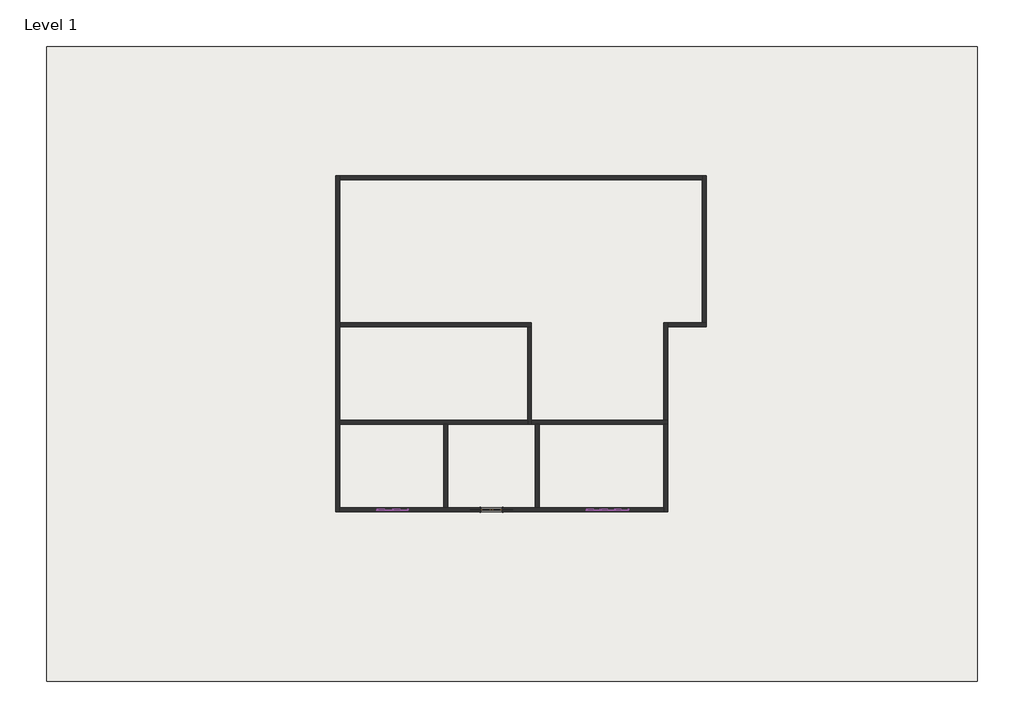
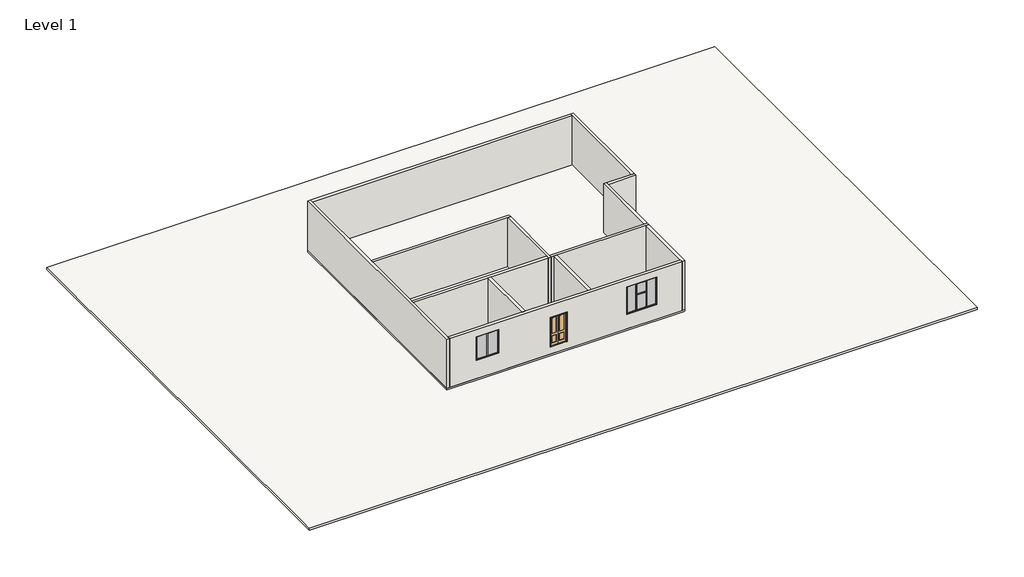
# One storey, incomplete: 22 members, 13 walls, 6 plates, 2 slabs, 1 door.
"""IFC4 building model written with IfcOpenShell, lengths in millimetres."""

from ifc_helpers import new_model, si_unit, frame, origin, origin_with_axes, place, context, project, spatial, polyline, outline, extrude, faceted_brep, transform, mapped, element, save
from components import door_interior_double_pocket_2_panel_wood_4_x_8_12c354ae, member_7007ad49, member_824a4a8d, member_798d6cad, member_9d02be77, member_c6627131, member_c17f1be2, member_f95d5bf5, member_18e22e2d, member_9193c932, member_0a82c195, system_panel_glazed_0771ef41, system_panel_glazed_b8cd24f7, system_panel_glazed_9a0fbd8e, system_panel_glazed_a3e6f34c

model = new_model("IFC4")

# Units and contexts
model_context = context("Model", 3, world=origin())
ifc_project = project(units=[si_unit("LENGTHUNIT", "METRE", prefix="MILLI")], contexts=[model_context])

# Site, building, storey
site = spatial("IfcSite", under=ifc_project)
building = spatial("IfcBuilding", under=site)
storey = spatial("IfcBuildingStorey", under=building, Name="Level 1", Elevation=0.0)

# Door
placement = place(None, origin())
door_interior_double_pocket_2_panel_wood_4_x_8_shape = door_interior_double_pocket_2_panel_wood_4_x_8_12c354ae(model_context)
element("IfcDoor", 1, ObjectType="Door-Interior-Double-Pocket-2_Panel-Wood : 4'x 8'", at=placement, inside=storey, context=model_context, shape_type="MappedRepresentation", body=[
    mapped(door_interior_double_pocket_2_panel_wood_4_x_8_shape, transform((-4678.5559085, -2978.2585517, 609.6), x_axis=(-1.0, 0.0, 0.0), y_axis=(0.0, -1.0, 0.0), z_axis=(0.0, 0.0, 1.0))),
])

# Members
member_shape = member_7007ad49(model_context)
element("IfcMember", 2, ObjectType="Rectangular Mullion : 2.5\" x 5\" rectangular", at=placement, inside=storey, context=model_context, shape_type="MappedRepresentation", body=[
    mapped(member_shape, transform((852.2940915, -2978.2585517, 3556.0), x_axis=(0.0, 0.0, 1.0), y_axis=(0.0, 1.0, 0.0), z_axis=(-1.0, 0.0, 0.0))),
])
element("IfcMember", 3, ObjectType="Rectangular Mullion : 2.5\" x 5\" rectangular", at=placement, inside=storey, context=model_context, shape_type="MappedRepresentation", body=[
    mapped(member_shape, transform((2446.1440915, -2978.2585517, 3556.0), x_axis=(0.0, 0.0, 1.0), y_axis=(0.0, 1.0, 0.0), z_axis=(-1.0, 0.0, 0.0))),
])
element("IfcMember", 4, ObjectType="Rectangular Mullion : 2.5\" x 5\" rectangular", at=placement, inside=storey, context=model_context, shape_type="MappedRepresentation", body=[
    mapped(member_shape, transform((3163.6940915, -2978.2585517, 1219.2), x_axis=(0.0, 0.0, -1.0), y_axis=(0.0, 1.0, 0.0), z_axis=(1.0, 0.0, 0.0))),
])
element("IfcMember", 5, ObjectType="Rectangular Mullion : 2.5\" x 5\" rectangular", at=placement, inside=storey, context=model_context, shape_type="MappedRepresentation", body=[
    mapped(member_shape, transform((1569.8440915, -2978.2585517, 1219.2), x_axis=(0.0, 0.0, -1.0), y_axis=(0.0, 1.0, 0.0), z_axis=(1.0, 0.0, 0.0))),
])
member_2_shape = member_824a4a8d(model_context)
element("IfcMember", 6, ObjectType="Rectangular Mullion : 2.5\" x 5\" rectangular", at=placement, inside=storey, context=model_context, shape_type="MappedRepresentation", body=[
    mapped(member_2_shape, transform((1601.5940915, -2978.2585517, 1219.2), x_axis=(-1.0, 0.0, 0.0), y_axis=(0.0, 1.0, 0.0), z_axis=(0.0, 0.0, -1.0))),
])
element("IfcMember", 7, ObjectType="Rectangular Mullion : 2.5\" x 5\" rectangular", at=placement, inside=storey, context=model_context, shape_type="MappedRepresentation", body=[
    mapped(member_2_shape, transform((2414.3940915, -2978.2585517, 1219.2), x_axis=(-1.0, 0.0, 0.0), y_axis=(0.0, 1.0, 0.0), z_axis=(0.0, 0.0, -1.0))),
])
member_3_shape = member_798d6cad(model_context)
element("IfcMember", 8, ObjectType="Rectangular Mullion : 2.5\" x 5\" rectangular", at=placement, inside=storey, context=model_context, shape_type="MappedRepresentation", body=[
    mapped(member_3_shape, transform((1633.3440915, -2978.2585517, 2590.8), x_axis=(0.0, 0.0, 1.0), y_axis=(0.0, 1.0, 0.0), z_axis=(-1.0, 0.0, 0.0))),
])
member_4_shape = member_9d02be77(model_context)
element("IfcMember", 9, ObjectType="Rectangular Mullion : 2.5\" x 5\" rectangular", at=placement, inside=storey, context=model_context, shape_type="MappedRepresentation", body=[
    mapped(member_4_shape, transform((2382.6440915, -2978.2585517, 1219.2), x_axis=(0.0, 0.0, -1.0), y_axis=(0.0, 1.0, 0.0), z_axis=(1.0, 0.0, 0.0))),
])
element("IfcMember", 10, ObjectType="Rectangular Mullion : 2.5\" x 5\" rectangular", at=placement, inside=storey, context=model_context, shape_type="MappedRepresentation", body=[
    mapped(member_4_shape, transform((1633.3440915, -2978.2585517, 3556.0), x_axis=(0.0, 0.0, 1.0), y_axis=(0.0, 1.0, 0.0), z_axis=(-1.0, 0.0, 0.0))),
])
member_5_shape = member_c6627131(model_context)
element("IfcMember", 11, ObjectType="Rectangular Mullion : 2.5\" x 5\" rectangular", at=placement, inside=storey, context=model_context, shape_type="MappedRepresentation", body=[
    mapped(member_5_shape, transform((788.7940915, -2978.2585517, 1219.2), x_axis=(-1.0, 0.0, 0.0), y_axis=(0.0, 1.0, 0.0), z_axis=(0.0, 0.0, -1.0))),
])
element("IfcMember", 12, ObjectType="Rectangular Mullion : 2.5\" x 5\" rectangular", at=placement, inside=storey, context=model_context, shape_type="MappedRepresentation", body=[
    mapped(member_5_shape, transform((3227.1940915, -2978.2585517, 2590.8), x_axis=(1.0, 0.0, 0.0), y_axis=(0.0, 1.0, 0.0), z_axis=(0.0, 0.0, 1.0))),
])
member_6_shape = member_c17f1be2(model_context)
element("IfcMember", 13, ObjectType="Rectangular Mullion : 2.5\" x 5\" rectangular", at=placement, inside=storey, context=model_context, shape_type="MappedRepresentation", body=[
    mapped(member_6_shape, transform((-11225.4059085, -2978.2585517, 3556.0), x_axis=(0.0, 0.0, 1.0), y_axis=(0.0, 1.0, 0.0), z_axis=(-1.0, 0.0, 0.0))),
])
element("IfcMember", 14, ObjectType="Rectangular Mullion : 2.5\" x 5\" rectangular", at=placement, inside=storey, context=model_context, shape_type="MappedRepresentation", body=[
    mapped(member_6_shape, transform((-10342.7559085, -2978.2585517, 3556.0), x_axis=(0.0, 0.0, 1.0), y_axis=(0.0, 1.0, 0.0), z_axis=(-1.0, 0.0, 0.0))),
])
element("IfcMember", 15, ObjectType="Rectangular Mullion : 2.5\" x 5\" rectangular", at=placement, inside=storey, context=model_context, shape_type="MappedRepresentation", body=[
    mapped(member_6_shape, transform((-9523.6059085, -2978.2585517, 1524.0), x_axis=(0.0, 0.0, -1.0), y_axis=(0.0, 1.0, 0.0), z_axis=(1.0, 0.0, 0.0))),
])
element("IfcMember", 16, ObjectType="Rectangular Mullion : 2.5\" x 5\" rectangular", at=placement, inside=storey, context=model_context, shape_type="MappedRepresentation", body=[
    mapped(member_6_shape, transform((-10406.2559085, -2978.2585517, 1524.0), x_axis=(0.0, 0.0, -1.0), y_axis=(0.0, 1.0, 0.0), z_axis=(1.0, 0.0, 0.0))),
])
member_7_shape = member_f95d5bf5(model_context)
element("IfcMember", 17, ObjectType="Rectangular Mullion : 2.5\" x 5\" rectangular", at=placement, inside=storey, context=model_context, shape_type="MappedRepresentation", body=[
    mapped(member_7_shape, transform((-10374.5059085, -2978.2585517, 1524.0), x_axis=(-1.0, 0.0, 0.0), y_axis=(0.0, 1.0, 0.0), z_axis=(0.0, 0.0, -1.0))),
])
member_8_shape = member_18e22e2d(model_context)
element("IfcMember", 18, ObjectType="Rectangular Mullion : 2.5\" x 5\" rectangular", at=placement, inside=storey, context=model_context, shape_type="MappedRepresentation", body=[
    mapped(member_8_shape, transform((1601.5940915, -2978.2585517, 2590.8), x_axis=(-1.0, 0.0, 0.0), y_axis=(0.0, 1.0, 0.0), z_axis=(0.0, 0.0, -1.0))),
])
element("IfcMember", 19, ObjectType="Rectangular Mullion : 2.5\" x 5\" rectangular", at=placement, inside=storey, context=model_context, shape_type="MappedRepresentation", body=[
    mapped(member_8_shape, transform((2414.3940915, -2978.2585517, 2590.8), x_axis=(-1.0, 0.0, 0.0), y_axis=(0.0, 1.0, 0.0), z_axis=(0.0, 0.0, -1.0))),
])
member_9_shape = member_9193c932(model_context)
element("IfcMember", 20, ObjectType="Rectangular Mullion : 2.5\" x 5\" rectangular", at=placement, inside=storey, context=model_context, shape_type="MappedRepresentation", body=[
    mapped(member_9_shape, transform((3227.1940915, -2978.2585517, 3556.0), x_axis=(1.0, 0.0, 0.0), y_axis=(0.0, 1.0, 0.0), z_axis=(0.0, 0.0, 1.0))),
])
element("IfcMember", 21, ObjectType="Rectangular Mullion : 2.5\" x 5\" rectangular", at=placement, inside=storey, context=model_context, shape_type="MappedRepresentation", body=[
    mapped(member_9_shape, transform((788.7940915, -2978.2585517, 2590.8), x_axis=(-1.0, 0.0, 0.0), y_axis=(0.0, 1.0, 0.0), z_axis=(0.0, 0.0, -1.0))),
])
member_10_shape = member_0a82c195(model_context)
element("IfcMember", 22, ObjectType="Rectangular Mullion : 2.5\" x 5\" rectangular", at=placement, inside=storey, context=model_context, shape_type="MappedRepresentation", body=[
    mapped(member_10_shape, transform((-9460.1059085, -2978.2585517, 3556.0), x_axis=(1.0, 0.0, 0.0), y_axis=(0.0, 1.0, 0.0), z_axis=(0.0, 0.0, 1.0))),
])
element("IfcMember", 23, ObjectType="Rectangular Mullion : 2.5\" x 5\" rectangular", at=placement, inside=storey, context=model_context, shape_type="MappedRepresentation", body=[
    mapped(member_10_shape, transform((-11288.9059085, -2978.2585517, 1524.0), x_axis=(-1.0, 0.0, 0.0), y_axis=(0.0, 1.0, 0.0), z_axis=(0.0, 0.0, -1.0))),
])

# Plates
system_panel_glazed_shape = system_panel_glazed_0771ef41(model_context)
element("IfcPlate", 24, ObjectType="System Panel : Glazed", at=placement, inside=storey, context=model_context, shape_type="MappedRepresentation", body=[
    mapped(system_panel_glazed_shape, transform((2007.9940915, -2978.2585517, 1282.7), x_axis=(-1.0, 0.0, 0.0), y_axis=(0.0, -1.0, 0.0), z_axis=(0.0, 0.0, 1.0))),
])
system_panel_glazed_2_shape = system_panel_glazed_b8cd24f7(model_context)
element("IfcPlate", 25, ObjectType="System Panel : Glazed", at=placement, inside=storey, context=model_context, shape_type="MappedRepresentation", body=[
    mapped(system_panel_glazed_2_shape, transform((-9933.1809085, -2978.2585517, 1587.5), x_axis=(-1.0, 0.0, 0.0), y_axis=(0.0, -1.0, 0.0), z_axis=(0.0, 0.0, 1.0))),
])
element("IfcPlate", 26, ObjectType="System Panel : Glazed", at=placement, inside=storey, context=model_context, shape_type="MappedRepresentation", body=[
    mapped(system_panel_glazed_2_shape, transform((-10815.8309085, -2978.2585517, 1587.5), x_axis=(-1.0, 0.0, 0.0), y_axis=(0.0, -1.0, 0.0), z_axis=(0.0, 0.0, 1.0))),
])
system_panel_glazed_3_shape = system_panel_glazed_9a0fbd8e(model_context)
element("IfcPlate", 27, ObjectType="System Panel : Glazed", at=placement, inside=storey, context=model_context, shape_type="MappedRepresentation", body=[
    mapped(system_panel_glazed_3_shape, transform((2804.9190915, -2978.2585517, 1282.7), x_axis=(-1.0, 0.0, 0.0), y_axis=(0.0, -1.0, 0.0), z_axis=(0.0, 0.0, 1.0))),
])
element("IfcPlate", 28, ObjectType="System Panel : Glazed", at=placement, inside=storey, context=model_context, shape_type="MappedRepresentation", body=[
    mapped(system_panel_glazed_3_shape, transform((1211.0690915, -2978.2585517, 1282.7), x_axis=(-1.0, 0.0, 0.0), y_axis=(0.0, -1.0, 0.0), z_axis=(0.0, 0.0, 1.0))),
])
system_panel_glazed_4_shape = system_panel_glazed_a3e6f34c(model_context)
element("IfcPlate", 29, ObjectType="System Panel : Glazed", at=placement, inside=storey, context=model_context, shape_type="MappedRepresentation", body=[
    mapped(system_panel_glazed_4_shape, transform((2007.9940915, -2978.2585517, 2622.55), x_axis=(-1.0, 0.0, 0.0), y_axis=(0.0, -1.0, 0.0), z_axis=(0.0, 0.0, 1.0))),
])

# Slabs
element("IfcSlab", 30, ObjectType="6\" floor", at=placement, inside=storey, context=model_context, shape_type="SweptSolid", body=[
    extrude(outline(polyline([(-13651.1059085, 16262.2414483), (7684.8940915, 16262.2414483), (7684.8940915, 7575.4414483), (5475.0940915, 7575.4414483), (5475.0940915, -3092.5585517), (-13651.1059085, -3092.5585517), (-13651.1059085, 16262.2414483)])), frame((0.0, 0.0, -152.4), z_axis=(0.0, 0.0, 1.0), x_axis=(1.0, 0.0, 0.0)), (0.0, 0.0, 1.0), 152.4),
])
element("IfcSlab", 31, ObjectType="6\" floor", at=placement, inside=storey, context=model_context, shape_type="SweptSolid", body=[
    extrude(outline(polyline([(23326.728978, 23712.5642574), (23326.728978, -12863.4357426), (-30318.071022, -12863.4357426), (-30318.071022, 23712.5642574), (23326.728978, 23712.5642574)])), frame((0.0, 0.0, -304.8), z_axis=(0.0, 0.0, 1.0), x_axis=(1.0, 0.0, 0.0)), (0.0, 0.0, 1.0), 152.4),
])

# Walls
element("IfcWall", 32, ObjectType="9\" wall", at=placement, inside=storey, context=model_context, shape_type="Brep", body=[
    faceted_brep([(-13651.1059085, 16262.2414483, 0.0), (-13651.1059085, -3092.5585517, 0.0), (-13651.1059085, -3092.5585517, 4165.6), (-13651.1059085, 16262.2414483, 4165.6), (-13422.5059085, 16262.2414483, 0.0), (-13422.5059085, 16262.2414483, 4165.6), (-13422.5059085, 16033.6414483, 4165.6), (-13422.5059085, 7804.0414483, 4165.6), (-13422.5059085, 7575.4414483, 4165.6), (-13422.5059085, 2165.2414483, 4165.6), (-13422.5059085, 1936.6414483, 4165.6), (-13422.5059085, -2863.9585517, 4165.6), (-13422.5059085, -3092.5585517, 4165.6), (-13422.5059085, -3092.5585517, 0.0), (-13422.5059085, -2863.9585517, 0.0), (-13422.5059085, 1936.6414483, 0.0), (-13422.5059085, 2165.2414483, 0.0), (-13422.5059085, 7575.4414483, 0.0), (-13422.5059085, 7804.0414483, 0.0), (-13422.5059085, 16033.6414483, 0.0)], [[[0, 1, 2, 3]], [[4, 5, 6, 7, 8, 9, 10, 11, 12, 13, 14, 15, 16, 17, 18, 19]], [[1, 0, 4, 19, 18, 17, 16, 15, 14, 13]], [[3, 2, 12, 11, 10, 9, 8, 7, 6, 5]], [[2, 1, 13, 12]], [[0, 3, 5, 4]]]),
])
element("IfcWall", 33, ObjectType="9\" wall", at=placement, inside=storey, context=model_context, shape_type="Brep", body=[
    faceted_brep([(-13422.5059085, 7575.4414483, 0.0), (-2602.1059085, 7575.4414483, 0.0), (-2373.5059085, 7575.4414483, 0.0), (-2373.5059085, 7575.4414483, 4165.6), (-2602.1059085, 7575.4414483, 4165.6), (-13422.5059085, 7575.4414483, 4165.6), (-13422.5059085, 7804.0414483, 0.0), (-13422.5059085, 7804.0414483, 4165.6), (-2373.5059085, 7804.0414483, 4165.6), (-2373.5059085, 7804.0414483, 0.0)], [[[0, 1, 2, 3, 4, 5]], [[6, 7, 8, 9]], [[2, 1, 0, 6, 9]], [[5, 4, 3, 8, 7]], [[0, 5, 7, 6]], [[3, 2, 9, 8]]]),
])
element("IfcWall", 34, ObjectType="9\" wall", at=placement, inside=storey, context=model_context, shape_type="Brep", body=[
    faceted_brep([(-2602.1059085, 7575.4414483, 0.0), (-2602.1059085, 2165.2414483, 0.0), (-2602.1059085, 1936.6414483, 0.0), (-2602.1059085, 1936.6414483, 4165.6), (-2602.1059085, 2165.2414483, 4165.6), (-2602.1059085, 7575.4414483, 4165.6), (-2373.5059085, 7575.4414483, 0.0), (-2373.5059085, 7575.4414483, 4165.6), (-2373.5059085, 2165.2414483, 4165.6), (-2373.5059085, 1936.6414483, 4165.6), (-2373.5059085, 1936.6414483, 0.0), (-2373.5059085, 2165.2414483, 0.0)], [[[0, 1, 2, 3, 4, 5]], [[6, 7, 8, 9, 10, 11]], [[2, 1, 0, 6, 11, 10]], [[5, 4, 3, 9, 8, 7]], [[0, 5, 7, 6]], [[3, 2, 10, 9]]]),
])
element("IfcWall", 35, ObjectType="9\" wall", at=placement, inside=storey, context=model_context, shape_type="Brep", body=[
    faceted_brep([(-2373.5059085, 1936.6414483, 0.0), (-2144.9059085, 1936.6414483, 0.0), (-1916.3059085, 1936.6414483, 0.0), (5246.4940915, 1936.6414483, 0.0), (5475.0940915, 1936.6414483, 0.0), (5475.0940915, 1936.6414483, 4165.6), (5246.4940915, 1936.6414483, 4165.6), (-1916.3059085, 1936.6414483, 4165.6), (-2144.9059085, 1936.6414483, 4165.6), (-2373.5059085, 1936.6414483, 4165.6), (-2373.5059085, 2165.2414483, 0.0), (-2373.5059085, 2165.2414483, 4165.6), (5246.4940915, 2165.2414483, 4165.6), (5475.0940915, 2165.2414483, 4165.6), (5475.0940915, 2165.2414483, 0.0), (5246.4940915, 2165.2414483, 0.0)], [[[0, 1, 2, 3, 4, 5, 6, 7, 8, 9]], [[10, 11, 12, 13, 14, 15]], [[4, 3, 2, 1, 0, 10, 15, 14]], [[9, 8, 7, 6, 5, 13, 12, 11]], [[0, 9, 11, 10]], [[5, 4, 14, 13]]]),
])
element("IfcWall", 36, ObjectType="9\" wall", at=placement, inside=storey, context=model_context, shape_type="Brep", body=[
    faceted_brep([(5475.0940915, 2165.2414483, 0.0), (5475.0940915, 7575.4414483, 0.0), (5475.0940915, 7804.0414483, 0.0), (5475.0940915, 7804.0414483, 4165.6), (5475.0940915, 7575.4414483, 4165.6), (5475.0940915, 2165.2414483, 4165.6), (5246.4940915, 2165.2414483, 0.0), (5246.4940915, 2165.2414483, 4165.6), (5246.4940915, 7804.0414483, 4165.6), (5246.4940915, 7804.0414483, 0.0)], [[[0, 1, 2, 3, 4, 5]], [[6, 7, 8, 9]], [[2, 1, 0, 6, 9]], [[5, 4, 3, 8, 7]], [[0, 5, 7, 6]], [[3, 2, 9, 8]]]),
])
element("IfcWall", 37, ObjectType="9\" wall", at=placement, inside=storey, context=model_context, shape_type="Brep", body=[
    faceted_brep([(-2602.1059085, 2165.2414483, 0.0), (-13422.5059085, 2165.2414483, 0.0), (-13422.5059085, 2165.2414483, 4165.6), (-2602.1059085, 2165.2414483, 4165.6), (-2602.1059085, 1936.6414483, 0.0), (-2602.1059085, 1936.6414483, 4165.6), (-7212.2059085, 1936.6414483, 4165.6), (-7440.8059085, 1936.6414483, 4165.6), (-13422.5059085, 1936.6414483, 4165.6), (-13422.5059085, 1936.6414483, 0.0), (-7440.8059085, 1936.6414483, 0.0), (-7212.2059085, 1936.6414483, 0.0)], [[[0, 1, 2, 3]], [[4, 5, 6, 7, 8, 9, 10, 11]], [[1, 0, 4, 11, 10, 9]], [[3, 2, 8, 7, 6, 5]], [[0, 3, 5, 4]], [[2, 1, 9, 8]]]),
])
element("IfcWall", 38, ObjectType="9\" wall", at=placement, inside=storey, context=model_context, shape_type="Brep", body=[
    faceted_brep([(5246.4940915, 1936.6414483, 0.0), (5246.4940915, -2863.9585517, 0.0), (5246.4940915, -3092.5585517, 0.0), (5246.4940915, -3092.5585517, 4165.6), (5246.4940915, -2863.9585517, 4165.6), (5246.4940915, 1936.6414483, 4165.6), (5475.0940915, 1936.6414483, 0.0), (5475.0940915, 1936.6414483, 4165.6), (5475.0940915, -3092.5585517, 4165.6), (5475.0940915, -3092.5585517, 0.0)], [[[0, 1, 2, 3, 4, 5]], [[6, 7, 8, 9]], [[2, 1, 0, 6, 9]], [[5, 4, 3, 8, 7]], [[0, 5, 7, 6]], [[3, 2, 9, 8]]]),
])
element("IfcWall", 39, ObjectType="9\" wall", at=placement, inside=storey, context=model_context, shape_type="Brep", body=[
    faceted_brep([(5246.4940915, -2863.9585517, 0.0), (-1916.3059085, -2863.9585517, 0.0), (-2144.9059085, -2863.9585517, 0.0), (-7212.2059085, -2863.9585517, 0.0), (-7440.8059085, -2863.9585517, 0.0), (-13422.5059085, -2863.9585517, 0.0), (-13422.5059085, -2863.9585517, 4165.6), (-7440.8059085, -2863.9585517, 4165.6), (-7212.2059085, -2863.9585517, 4165.6), (-2144.9059085, -2863.9585517, 4165.6), (-1916.3059085, -2863.9585517, 4165.6), (5246.4940915, -2863.9585517, 4165.6), (-4043.5559085, -2863.9585517, 3073.4), (-5313.5559085, -2863.9585517, 3073.4), (-5313.5559085, -2863.9585517, 609.6), (-4043.5559085, -2863.9585517, 609.6), (-9460.1059085, -2863.9585517, 1524.0), (-9460.1059085, -2863.9585517, 3556.0), (-11288.9059085, -2863.9585517, 3556.0), (-11288.9059085, -2863.9585517, 1524.0), (3227.1940915, -2863.9585517, 1219.2), (3227.1940915, -2863.9585517, 3556.0), (788.7940915, -2863.9585517, 3556.0), (788.7940915, -2863.9585517, 1219.2), (-13422.5059085, -3092.5585517, 0.0), (5246.4940915, -3092.5585517, 0.0), (5246.4940915, -3092.5585517, 4165.6), (-13422.5059085, -3092.5585517, 4165.6), (-5313.5559085, -3092.5585517, 3073.4), (-4043.5559085, -3092.5585517, 3073.4), (-4043.5559085, -3092.5585517, 609.6), (-5313.5559085, -3092.5585517, 609.6), (-9460.1059085, -3092.5585517, 3556.0), (-9460.1059085, -3092.5585517, 1524.0), (-11288.9059085, -3092.5585517, 1524.0), (-11288.9059085, -3092.5585517, 3556.0), (3227.1940915, -3092.5585517, 3556.0), (3227.1940915, -3092.5585517, 1219.2), (788.7940915, -3092.5585517, 1219.2), (788.7940915, -3092.5585517, 3556.0), (-5923.1559085, -2998.8960517, 3073.4), (-5923.1559085, -2957.6210517, 3073.4), (-5313.5559085, -2957.6210517, 3073.4), (-4043.5559085, -2957.6210517, 3073.4), (-3433.9559085, -2957.6210517, 3073.4), (-3433.9559085, -2998.8960517, 3073.4), (-4043.5559085, -2998.8960517, 3073.4), (-5313.5559085, -2998.8960517, 3073.4), (-5923.1559085, -2998.8960517, 609.6), (-5313.5559085, -2998.8960517, 609.6), (-4043.5559085, -2998.8960517, 609.6), (-3433.9559085, -2998.8960517, 609.6), (-3433.9559085, -2957.6210517, 609.6), (-4043.5559085, -2957.6210517, 609.6), (-5313.5559085, -2957.6210517, 609.6), (-5923.1559085, -2957.6210517, 609.6)], [[[0, 1, 2, 3, 4, 5, 6, 7, 8, 9, 10, 11], [12, 13, 14, 15], [16, 17, 18, 19], [20, 21, 22, 23]], [[24, 25, 26, 27], [28, 29, 30, 31], [32, 33, 34, 35], [36, 37, 38, 39]], [[5, 4, 3, 2, 1, 0, 25, 24]], [[11, 10, 9, 8, 7, 6, 27, 26]], [[0, 11, 26, 25]], [[6, 5, 24, 27]], [[40, 41, 42, 13, 12, 43, 44, 45, 46, 29, 28, 47]], [[48, 49, 31, 30, 50, 51, 52, 53, 15, 14, 54, 55]], [[40, 47, 49, 48]], [[47, 28, 31, 49]], [[29, 46, 50, 30]], [[46, 45, 51, 50]], [[45, 44, 52, 51]], [[44, 43, 53, 52]], [[43, 12, 15, 53]], [[13, 42, 54, 14]], [[42, 41, 55, 54]], [[41, 40, 48, 55]], [[32, 17, 16, 33]], [[17, 32, 35, 18]], [[18, 35, 34, 19]], [[33, 16, 19, 34]], [[36, 21, 20, 37]], [[21, 36, 39, 22]], [[22, 39, 38, 23]], [[37, 20, 23, 38]]]),
])
element("IfcWall", 40, ObjectType="9\" wall", at=placement, inside=storey, context=model_context, shape_type="SweptSolid", body=[
    extrude(outline(polyline([(-1916.3059085, 1936.6414483), (-1916.3059085, -2863.9585517), (-2144.9059085, -2863.9585517), (-2144.9059085, 1936.6414483), (-1916.3059085, 1936.6414483)])), origin_with_axes(), (0.0, 0.0, 1.0), 4165.6),
])
element("IfcWall", 41, ObjectType="9\" wall", at=placement, inside=storey, context=model_context, shape_type="SweptSolid", body=[
    extrude(outline(polyline([(-7440.8059085, -2863.9585517), (-7440.8059085, 1936.6414483), (-7212.2059085, 1936.6414483), (-7212.2059085, -2863.9585517), (-7440.8059085, -2863.9585517)])), origin_with_axes(), (0.0, 0.0, 1.0), 4165.6),
])
element("IfcWall", 42, ObjectType="9\" wall", at=placement, inside=storey, context=model_context, shape_type="Brep", body=[
    faceted_brep([(5475.0940915, 7575.4414483, 0.0), (7684.8940915, 7575.4414483, 0.0), (7684.8940915, 7575.4414483, 4165.6), (5475.0940915, 7575.4414483, 4165.6), (5475.0940915, 7804.0414483, 0.0), (5475.0940915, 7804.0414483, 4165.6), (7456.2940915, 7804.0414483, 4165.6), (7684.8940915, 7804.0414483, 4165.6), (7684.8940915, 7804.0414483, 0.0), (7456.2940915, 7804.0414483, 0.0)], [[[0, 1, 2, 3]], [[4, 5, 6, 7, 8, 9]], [[1, 0, 4, 9, 8]], [[3, 2, 7, 6, 5]], [[0, 3, 5, 4]], [[2, 1, 8, 7]]]),
])
element("IfcWall", 43, ObjectType="9\" wall", at=placement, inside=storey, context=model_context, shape_type="Brep", body=[
    faceted_brep([(7684.8940915, 7804.0414483, 0.0), (7684.8940915, 16262.2414483, 0.0), (7684.8940915, 16262.2414483, 4165.6), (7684.8940915, 7804.0414483, 4165.6), (7456.2940915, 7804.0414483, 0.0), (7456.2940915, 7804.0414483, 4165.6), (7456.2940915, 16033.6414483, 4165.6), (7456.2940915, 16262.2414483, 4165.6), (7456.2940915, 16262.2414483, 0.0), (7456.2940915, 16033.6414483, 0.0)], [[[0, 1, 2, 3]], [[4, 5, 6, 7, 8, 9]], [[1, 0, 4, 9, 8]], [[3, 2, 7, 6, 5]], [[0, 3, 5, 4]], [[2, 1, 8, 7]]]),
])
element("IfcWall", 44, ObjectType="9\" wall", at=placement, inside=storey, context=model_context, shape_type="SweptSolid", body=[
    extrude(outline(polyline([(-13422.5059085, 16262.2414483), (7456.2940915, 16262.2414483), (7456.2940915, 16033.6414483), (-13422.5059085, 16033.6414483), (-13422.5059085, 16262.2414483)])), origin_with_axes(), (0.0, 0.0, 1.0), 4165.6),
])

save(model, "model.ifc")

# Revit data of these elements
# Type "Door-Interior-Double-Pocket-2_Panel-Wood : 4'x 8'"
#   Type Mark = "9"
#   Assembly Code = "C1020300"
#   Analytic Construction = "Wooden"
#   Top Rail = 0' - 4 11/16"
#   Thickness = 0' - 1 3/8"
#   Thermal Resistance (R) = 2.5876 (h·ft²·°F)/BTU
#   Stiles = 0' - 4 3/4"
#   Rough Width = 8' - 2"
#   Rough Height = 8' - 4 1/2"
#   Panel Width = 2' - 0"
#   Lock Rail = 0' - 7 1/2"
#   Location [instance default] = 2' - 1"
#   Height = 8' - 0"
#   Width = 4' - 0"
#   Heat Transfer Coefficient (U) = 0.3865 BTU/(h·ft²·°F)
#   Bottom Rail = 0' - 9 1/8"
#   Panel Open [instance default] = no
#   Trim Material = Cherry
#   Panel Material = wood door
#   Frame Material = Cherry
#   Visual Light Transmittance = 0
#   Solar Heat Gain Coefficient = 0
#   Wall Closure = (empty or 0)
#   Function = (empty or 0)
# Type "Rectangular Mullion : 2.5\" x 5\" rectangular"
#   built-in parameter 1007304 = 0.416667 (stored number, unit not read)
#   built-in parameter 1007301 = 0.104167 (stored number, unit not read)
#   built-in parameter 1007300 = 0.104167 (stored number, unit not read)
# Type "System Panel : Glazed"
#   Construction Type Id = "GSP4R"
#   Analytic Construction = "1/8 in Pilkington single glazing"
#   Visual Light Transmittance = 0.9
#   Solar Heat Gain Coefficient = 0.86
#   Heat Transfer Coefficient (U) = 1.18115 BTU/(h·ft²·°F)
#   Define Thermal Properties by = 1
# Type "6\" floor"
#   Assembly Code = "B1010"
#   Function = 0
#   Layers, outside or top first: 0' - 6" "floor" (function 1)
# Type "9\" wall"
#   Assembly Code = "B2010"
#   Layers, outside or top first: 0' - 9" "warm colour" (function 1)
# Element 1 (IfcDoor, "Door-Interior-Double-Pocket-2_Panel-Wood : 4'x 8'")
#   Location = 2' - 1"
#   Panel Open = no
#   Phase Created = New Construction
#   Materials on its faces: "wood door", "Cherry"
# Elements 2, 3, 4, 5, 6, 7, 8, 9, 10, 11, 12, 13, 14, 15, 16, 17, 18, 19, 20, 21, 22, 23 (IfcMember, "Rectangular Mullion : 2.5\" x 5\" rectangular")
#   Phase Created = New Construction
# Elements 24, 25, 26, 27, 28, 29 (IfcPlate, "System Panel : Glazed")
#   Phase Created = New Construction
#   Materials on its faces: "Glass"
# Element 30 (IfcSlab, "6\" floor")
#   built-in parameter 1001955 = 3.14159 (stored number, unit not read)
#   Height Offset From Level = 0' - 0"
#   Phase Created = New Construction
#   Materials on its faces: "floor"
# Element 31 (IfcSlab, "6\" floor")
#   Height Offset From Level = -0' - 6"
#   Phase Created = New Construction
#   Materials on its faces: "floor"
# Elements 32, 33, 34, 35, 36, 37, 38, 39, 40, 41, 42, 43, 44 (IfcWall, "9\" wall")
#   Top Offset = 0' - 0"
#   Base Offset = 0' - 0"
#   wall height = 13' - 8"
#   Phase Created = New Construction
#   Base Constraint = Level 1
#   Top Constraint = Level 2
#   Materials on its faces: "warm colour"
# Materials
#   "Cherry": class "Wood", colour RGB 226 177 128, transparency 0, Description = "Prunus Serotina", Cost = 0
#   "wood door": class "Generic", colour RGB 120 120 120, transparency 0, Cost = 0
#   "floor": class "Generic", colour RGB 120 120 120, transparency 0, Cost = 0
#   "warm colour": class "Generic", colour RGB 120 120 120, transparency 0, Cost = 0
#   "Glass": class "Glass", colour RGB 0 128 192, transparency 0.75, Description = "Soda Lime Glass", Cost = 0
